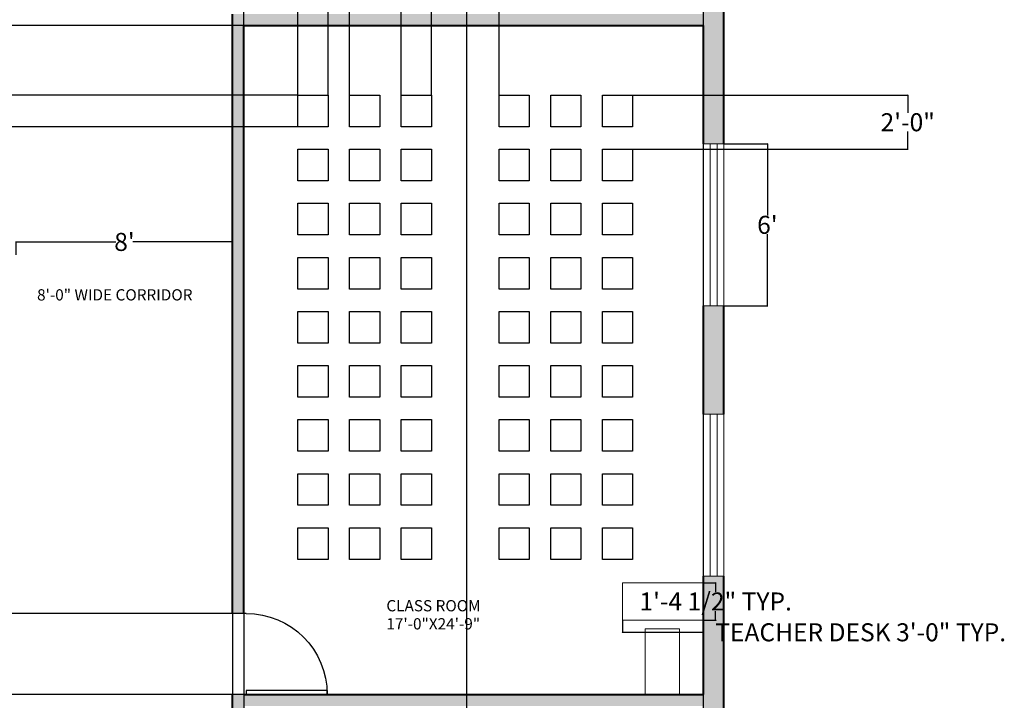
# Model space of a CAD drawing. Units: inches. Extents: x -405 to 940, y 226 to 2032.
# Tile 9 of 10: x 503 to 940, y 1301 to 1603. Entities that reach past the tile are written whole.
import ezdxf

# ---------------------------------------------------------------- set-up
doc = ezdxf.new("R2010")
doc.units = ezdxf.units.IN
doc.header["$MEASUREMENT"] = 0
doc.linetypes.add('ACAD_ISO02W100', pattern=[15, 12, -3])
for name, color, linetype, lineweight in [('A-ANNO-DIMS', 120, 'Continuous', 18), ('A-AREA-IDEN', 32, 'Continuous', 18), ('A-FURN-SEAT', 5, 'Continuous', 18), ('A-GLAZ-HIDN', 1, 'ACAD_ISO02W100', 18), ('A-WALL-PATT', 8, 'Continuous', 13), ('door', 6, 'Continuous', 25), ('tables', 2, 'Continuous', 18), ('wall', 3, 'Continuous', 40), ('window', 1, 'Continuous', 18)]:
    doc.layers.add(name, color=color, linetype=linetype, lineweight=lineweight)
doc.layers.add('beches', color=5, linetype='Continuous')
doc.styles.get("Standard").update_dxf_attribs({"font": 'arial.ttf'})
doc.dimstyles.get("Standard").update_dxf_attribs({"dimtxt": 8, "dimasz": 0.18, "dimexe": 0.18, "dimexo": 0.0625, "dimgap": 0.09, "dimtad": 0, "dimtih": 1, "dimtoh": 1, "dimdec": 0, "dimzin": 0, "dimdsep": 46, "dimlunit": 3, "dimtxsty": 'Standard', "dimblk": 'OBLIQUE', "dimcen": 0.09, "dimadec": 0, "dimazin": 0, "dimtfac": 1, "dimtdec": 0, "dimtofl": 0, "dimtmove": 0, "dimatfit": 3, "dimfxl": 1, "dimtolj": 1, "dimtzin": 0, "dimarcsym": 0})

# ---------------------------------------------------------------- blocks, each defined once
blk = doc.blocks.new('*U4')
for p, q in [((0, 0), (0, -6)), ((36, 0), (36, -6))]:
    blk.add_line(p, q)
blk.add_lwpolyline([(0, 0), (0, 36), (1.75, 36), (1.75, 0)], close=True)
blk.add_arc((0, 0), 36, 0, 90)
blk = doc.blocks.new('*U25')
at = {"layer": 'beches'}
blk.add_lwpolyline([(6.71, -7.02), (-6.71, -7.02), (-6.71, 7.02), (6.71, 7.02)], close=True, dxfattribs=at)
blk = doc.blocks.new('*U26')
at = {"layer": 'A-FURN-SEAT', "transparency": 16777216}
for p in [(-45.84, 192), (-45.84, 192, 12), (-45.84, 192, 24), (-45.84, 192, 36), (-45.84, 192, 48), (-45.84, 192, 60), (-45.84, 192, 72), (-45.84, 192, 84), (-45.84, 192, 96), (-45.84, 192, 108), (-45.84, 192, 120), (-45.84, 192, 132), (-22.92, 192), (-22.92, 192, 12), (-22.92, 192, 24), (-22.92, 192, 36), (-22.92, 192, 48), (-22.92, 192, 60), (-22.92, 192, 72), (-22.92, 192, 84), (-22.92, 192, 96), (-22.92, 192, 108), (-22.92, 192, 120), (-22.92, 192, 132), (0, 192), (0, 192, 12), (0, 192, 24), (0, 192, 36), (0, 192, 48), (0, 192, 60), (0, 192, 72), (0, 192, 84), (0, 192, 96), (0, 192, 108), (0, 192, 120), (0, 192, 132), (-45.84, 168), (-45.84, 168, 12), (-45.84, 168, 24), (-45.84, 168, 36), (-45.84, 168, 48), (-45.84, 168, 60), (-45.84, 168, 72), (-45.84, 168, 84), (-45.84, 168, 96), (-45.84, 168, 108), (-45.84, 168, 120), (-45.84, 168, 132), (-22.92, 168), (-22.92, 168, 12), (-22.92, 168, 24), (-22.92, 168, 36), (-22.92, 168, 48), (-22.92, 168, 60), (-22.92, 168, 72), (-22.92, 168, 84), (-22.92, 168, 96), (-22.92, 168, 108), (-22.92, 168, 120), (-22.92, 168, 132), (0, 168), (0, 168, 12), (0, 168, 24), (0, 168, 36), (0, 168, 48), (0, 168, 60), (0, 168, 72), (0, 168, 84), (0, 168, 96), (0, 168, 108), (0, 168, 120), (0, 168, 132), (-45.84, 144), (-45.84, 144, 12), (-45.84, 144, 24), (-45.84, 144, 36), (-45.84, 144, 48), (-45.84, 144, 60), (-45.84, 144, 72), (-45.84, 144, 84), (-45.84, 144, 96), (-45.84, 144, 108), (-45.84, 144, 120), (-45.84, 144, 132), (-22.92, 144), (-22.92, 144, 12), (-22.92, 144, 24), (-22.92, 144, 36), (-22.92, 144, 48), (-22.92, 144, 60), (-22.92, 144, 72), (-22.92, 144, 84), (-22.92, 144, 96), (-22.92, 144, 108), (-22.92, 144, 120), (-22.92, 144, 132), (0, 144), (0, 144, 12), (0, 144, 24), (0, 144, 36), (0, 144, 48), (0, 144, 60), (0, 144, 72), (0, 144, 84), (0, 144, 96), (0, 144, 108), (0, 144, 120), (0, 144, 132), (-45.84, 120), (-45.84, 120, 12), (-45.84, 120, 24), (-45.84, 120, 36), (-45.84, 120, 48), (-45.84, 120, 60), (-45.84, 120, 72), (-45.84, 120, 84), (-45.84, 120, 96), (-45.84, 120, 108), (-45.84, 120, 120), (-45.84, 120, 132), (-22.92, 120), (-22.92, 120, 12), (-22.92, 120, 24), (-22.92, 120, 36), (-22.92, 120, 48), (-22.92, 120, 60), (-22.92, 120, 72), (-22.92, 120, 84), (-22.92, 120, 96), (-22.92, 120, 108), (-22.92, 120, 120), (-22.92, 120, 132), (0, 120), (0, 120, 12), (0, 120, 24), (0, 120, 36), (0, 120, 48), (0, 120, 60), (0, 120, 72), (0, 120, 84), (0, 120, 96), (0, 120, 108), (0, 120, 120), (0, 120, 132), (-45.84, 96), (-45.84, 96, 12), (-45.84, 96, 24), (-45.84, 96, 36), (-45.84, 96, 48), (-45.84, 96, 60), (-45.84, 96, 72), (-45.84, 96, 84), (-45.84, 96, 96), (-45.84, 96, 108), (-45.84, 96, 120), (-45.84, 96, 132), (-22.92, 96), (-22.92, 96, 12), (-22.92, 96, 24), (-22.92, 96, 36), (-22.92, 96, 48), (-22.92, 96, 60), (-22.92, 96, 72), (-22.92, 96, 84), (-22.92, 96, 96), (-22.92, 96, 108), (-22.92, 96, 120), (-22.92, 96, 132), (0, 96), (0, 96, 12), (0, 96, 24), (0, 96, 36), (0, 96, 48), (0, 96, 60), (0, 96, 72), (0, 96, 84), (0, 96, 96), (0, 96, 108), (0, 96, 120), (0, 96, 132), (-45.84, 72), (-45.84, 72, 12), (-45.84, 72, 24), (-45.84, 72, 36), (-45.84, 72, 48), (-45.84, 72, 60), (-45.84, 72, 72), (-45.84, 72, 84), (-45.84, 72, 96), (-45.84, 72, 108), (-45.84, 72, 120), (-45.84, 72, 132), (-22.92, 72), (-22.92, 72, 12), (-22.92, 72, 24), (-22.92, 72, 36), (-22.92, 72, 48), (-22.92, 72, 60), (-22.92, 72, 72), (-22.92, 72, 84), (-22.92, 72, 96), (-22.92, 72, 108), (-22.92, 72, 120), (-22.92, 72, 132), (0, 72), (0, 72, 12), (0, 72, 24), (0, 72, 36), (0, 72, 48), (0, 72, 60), (0, 72, 72), (0, 72, 84), (0, 72, 96), (0, 72, 108), (0, 72, 120), (0, 72, 132), (-45.84, 48), (-45.84, 48, 12), (-45.84, 48, 24), (-45.84, 48, 36), (-45.84, 48, 48), (-45.84, 48, 60), (-45.84, 48, 72), (-45.84, 48, 84), (-45.84, 48, 96), (-45.84, 48, 108), (-45.84, 48, 120), (-45.84, 48, 132), (-22.92, 48), (-22.92, 48, 12), (-22.92, 48, 24), (-22.92, 48, 36), (-22.92, 48, 48), (-22.92, 48, 60), (-22.92, 48, 72), (-22.92, 48, 84), (-22.92, 48, 96), (-22.92, 48, 108), (-22.92, 48, 120), (-22.92, 48, 132), (0, 48), (0, 48, 12), (0, 48, 24), (0, 48, 36), (0, 48, 48), (0, 48, 60), (0, 48, 72), (0, 48, 84), (0, 48, 96), (0, 48, 108), (0, 48, 120), (0, 48, 132), (-45.84, 24), (-45.84, 24, 12), (-45.84, 24, 24), (-45.84, 24, 36), (-45.84, 24, 48), (-45.84, 24, 60), (-45.84, 24, 72), (-45.84, 24, 84), (-45.84, 24, 96), (-45.84, 24, 108), (-45.84, 24, 120), (-45.84, 24, 132), (-22.92, 24), (-22.92, 24, 12), (-22.92, 24, 24), (-22.92, 24, 36), (-22.92, 24, 48), (-22.92, 24, 60), (-22.92, 24, 72), (-22.92, 24, 84), (-22.92, 24, 96), (-22.92, 24, 108), (-22.92, 24, 120), (-22.92, 24, 132), (0, 24), (0, 24, 12), (0, 24, 24), (0, 24, 36), (0, 24, 48), (0, 24, 60), (0, 24, 72), (0, 24, 84), (0, 24, 96), (0, 24, 108), (0, 24, 120), (0, 24, 132), (-45.84, 0), (-45.84, 0, 12), (-45.84, 0, 24), (-45.84, 0, 36), (-45.84, 0, 48), (-45.84, 0, 60), (-45.84, 0, 72), (-45.84, 0, 84), (-45.84, 0, 96), (-45.84, 0, 108), (-45.84, 0, 120), (-45.84, 0, 132), (-22.92, 0), (-22.92, 0, 12), (-22.92, 0, 24), (-22.92, 0, 36), (-22.92, 0, 48), (-22.92, 0, 60), (-22.92, 0, 72), (-22.92, 0, 84), (-22.92, 0, 96), (-22.92, 0, 108), (-22.92, 0, 120), (-22.92, 0, 132), (0, 0), (0, 0, 12), (0, 0, 24), (0, 0, 36), (0, 0, 48), (0, 0, 60), (0, 0, 72), (0, 0, 84), (0, 0, 96), (0, 0, 108), (0, 0, 120), (0, 0, 132)]:
    blk.add_blockref('*U25', p, dxfattribs=at)
blk = doc.blocks.new('*U23')
at = {"layer": 'beches'}
blk.add_lwpolyline([(6.71, -7.02), (-6.71, -7.02), (-6.71, 7.02), (6.71, 7.02)], close=True, dxfattribs=at)
blk = doc.blocks.new('*U24')
at = {"layer": 'A-FURN-SEAT', "transparency": 16777216}
for p in [(-45.84, 192), (-45.84, 192, 12), (-45.84, 192, 24), (-45.84, 192, 36), (-45.84, 192, 48), (-45.84, 192, 60), (-45.84, 192, 72), (-45.84, 192, 84), (-45.84, 192, 96), (-45.84, 192, 108), (-45.84, 192, 120), (-45.84, 192, 132), (-22.92, 192), (-22.92, 192, 12), (-22.92, 192, 24), (-22.92, 192, 36), (-22.92, 192, 48), (-22.92, 192, 60), (-22.92, 192, 72), (-22.92, 192, 84), (-22.92, 192, 96), (-22.92, 192, 108), (-22.92, 192, 120), (-22.92, 192, 132), (0, 192), (0, 192, 12), (0, 192, 24), (0, 192, 36), (0, 192, 48), (0, 192, 60), (0, 192, 72), (0, 192, 84), (0, 192, 96), (0, 192, 108), (0, 192, 120), (0, 192, 132), (-45.84, 168), (-45.84, 168, 12), (-45.84, 168, 24), (-45.84, 168, 36), (-45.84, 168, 48), (-45.84, 168, 60), (-45.84, 168, 72), (-45.84, 168, 84), (-45.84, 168, 96), (-45.84, 168, 108), (-45.84, 168, 120), (-45.84, 168, 132), (-22.92, 168), (-22.92, 168, 12), (-22.92, 168, 24), (-22.92, 168, 36), (-22.92, 168, 48), (-22.92, 168, 60), (-22.92, 168, 72), (-22.92, 168, 84), (-22.92, 168, 96), (-22.92, 168, 108), (-22.92, 168, 120), (-22.92, 168, 132), (0, 168), (0, 168, 12), (0, 168, 24), (0, 168, 36), (0, 168, 48), (0, 168, 60), (0, 168, 72), (0, 168, 84), (0, 168, 96), (0, 168, 108), (0, 168, 120), (0, 168, 132), (-45.84, 144), (-45.84, 144, 12), (-45.84, 144, 24), (-45.84, 144, 36), (-45.84, 144, 48), (-45.84, 144, 60), (-45.84, 144, 72), (-45.84, 144, 84), (-45.84, 144, 96), (-45.84, 144, 108), (-45.84, 144, 120), (-45.84, 144, 132), (-22.92, 144), (-22.92, 144, 12), (-22.92, 144, 24), (-22.92, 144, 36), (-22.92, 144, 48), (-22.92, 144, 60), (-22.92, 144, 72), (-22.92, 144, 84), (-22.92, 144, 96), (-22.92, 144, 108), (-22.92, 144, 120), (-22.92, 144, 132), (0, 144), (0, 144, 12), (0, 144, 24), (0, 144, 36), (0, 144, 48), (0, 144, 60), (0, 144, 72), (0, 144, 84), (0, 144, 96), (0, 144, 108), (0, 144, 120), (0, 144, 132), (-45.84, 120), (-45.84, 120, 12), (-45.84, 120, 24), (-45.84, 120, 36), (-45.84, 120, 48), (-45.84, 120, 60), (-45.84, 120, 72), (-45.84, 120, 84), (-45.84, 120, 96), (-45.84, 120, 108), (-45.84, 120, 120), (-45.84, 120, 132), (-22.92, 120), (-22.92, 120, 12), (-22.92, 120, 24), (-22.92, 120, 36), (-22.92, 120, 48), (-22.92, 120, 60), (-22.92, 120, 72), (-22.92, 120, 84), (-22.92, 120, 96), (-22.92, 120, 108), (-22.92, 120, 120), (-22.92, 120, 132), (0, 120), (0, 120, 12), (0, 120, 24), (0, 120, 36), (0, 120, 48), (0, 120, 60), (0, 120, 72), (0, 120, 84), (0, 120, 96), (0, 120, 108), (0, 120, 120), (0, 120, 132), (-45.84, 96), (-45.84, 96, 12), (-45.84, 96, 24), (-45.84, 96, 36), (-45.84, 96, 48), (-45.84, 96, 60), (-45.84, 96, 72), (-45.84, 96, 84), (-45.84, 96, 96), (-45.84, 96, 108), (-45.84, 96, 120), (-45.84, 96, 132), (-22.92, 96), (-22.92, 96, 12), (-22.92, 96, 24), (-22.92, 96, 36), (-22.92, 96, 48), (-22.92, 96, 60), (-22.92, 96, 72), (-22.92, 96, 84), (-22.92, 96, 96), (-22.92, 96, 108), (-22.92, 96, 120), (-22.92, 96, 132), (0, 96), (0, 96, 12), (0, 96, 24), (0, 96, 36), (0, 96, 48), (0, 96, 60), (0, 96, 72), (0, 96, 84), (0, 96, 96), (0, 96, 108), (0, 96, 120), (0, 96, 132), (-45.84, 72), (-45.84, 72, 12), (-45.84, 72, 24), (-45.84, 72, 36), (-45.84, 72, 48), (-45.84, 72, 60), (-45.84, 72, 72), (-45.84, 72, 84), (-45.84, 72, 96), (-45.84, 72, 108), (-45.84, 72, 120), (-45.84, 72, 132), (-22.92, 72), (-22.92, 72, 12), (-22.92, 72, 24), (-22.92, 72, 36), (-22.92, 72, 48), (-22.92, 72, 60), (-22.92, 72, 72), (-22.92, 72, 84), (-22.92, 72, 96), (-22.92, 72, 108), (-22.92, 72, 120), (-22.92, 72, 132), (0, 72), (0, 72, 12), (0, 72, 24), (0, 72, 36), (0, 72, 48), (0, 72, 60), (0, 72, 72), (0, 72, 84), (0, 72, 96), (0, 72, 108), (0, 72, 120), (0, 72, 132), (-45.84, 48), (-45.84, 48, 12), (-45.84, 48, 24), (-45.84, 48, 36), (-45.84, 48, 48), (-45.84, 48, 60), (-45.84, 48, 72), (-45.84, 48, 84), (-45.84, 48, 96), (-45.84, 48, 108), (-45.84, 48, 120), (-45.84, 48, 132), (-22.92, 48), (-22.92, 48, 12), (-22.92, 48, 24), (-22.92, 48, 36), (-22.92, 48, 48), (-22.92, 48, 60), (-22.92, 48, 72), (-22.92, 48, 84), (-22.92, 48, 96), (-22.92, 48, 108), (-22.92, 48, 120), (-22.92, 48, 132), (0, 48), (0, 48, 12), (0, 48, 24), (0, 48, 36), (0, 48, 48), (0, 48, 60), (0, 48, 72), (0, 48, 84), (0, 48, 96), (0, 48, 108), (0, 48, 120), (0, 48, 132), (-45.84, 24), (-45.84, 24, 12), (-45.84, 24, 24), (-45.84, 24, 36), (-45.84, 24, 48), (-45.84, 24, 60), (-45.84, 24, 72), (-45.84, 24, 84), (-45.84, 24, 96), (-45.84, 24, 108), (-45.84, 24, 120), (-45.84, 24, 132), (-22.92, 24), (-22.92, 24, 12), (-22.92, 24, 24), (-22.92, 24, 36), (-22.92, 24, 48), (-22.92, 24, 60), (-22.92, 24, 72), (-22.92, 24, 84), (-22.92, 24, 96), (-22.92, 24, 108), (-22.92, 24, 120), (-22.92, 24, 132), (0, 24), (0, 24, 12), (0, 24, 24), (0, 24, 36), (0, 24, 48), (0, 24, 60), (0, 24, 72), (0, 24, 84), (0, 24, 96), (0, 24, 108), (0, 24, 120), (0, 24, 132), (-45.84, 0), (-45.84, 0, 12), (-45.84, 0, 24), (-45.84, 0, 36), (-45.84, 0, 48), (-45.84, 0, 60), (-45.84, 0, 72), (-45.84, 0, 84), (-45.84, 0, 96), (-45.84, 0, 108), (-45.84, 0, 120), (-45.84, 0, 132), (-22.92, 0), (-22.92, 0, 12), (-22.92, 0, 24), (-22.92, 0, 36), (-22.92, 0, 48), (-22.92, 0, 60), (-22.92, 0, 72), (-22.92, 0, 84), (-22.92, 0, 96), (-22.92, 0, 108), (-22.92, 0, 120), (-22.92, 0, 132), (0, 0), (0, 0, 12), (0, 0, 24), (0, 0, 36), (0, 0, 48), (0, 0, 60), (0, 0, 72), (0, 0, 84), (0, 0, 96), (0, 0, 108), (0, 0, 120), (0, 0, 132)]:
    blk.add_blockref('*U23', p, dxfattribs=at)
blk = doc.blocks.new('_Oblique')
at = {"color": 0, "linetype": 'ByBlock', "lineweight": -2}
blk.add_line((-0.5, -0.5), (0.5, 0.5), dxfattribs=at)
blk = doc.blocks.new('*D42')
at = {"layer": 'A-ANNO-DIMS', "color": 0, "lineweight": -2, "transparency": 16777216}
for p, q in [((501.77, 1498.93), (501.77, 1504.9)), ((501.77, 1504.72), (545.99, 1504.72)), ((597.77, 1504.72), (553.54, 1504.72)), ((597.77, 1498.93), (597.77, 1504.9))]:
    blk.add_line(p, q, dxfattribs=at)
at = {"layer": 'Defpoints', "color": 0, "transparency": 16777216}
for p in [(501.77, 1504.72), (501.77, 1498.87), (597.77, 1498.87)]:
    blk.add_point(p, dxfattribs=at)
at = {"layer": 'A-ANNO-DIMS', "color": 0, "lineweight": -2, "transparency": 16777216, "xscale": 0.18, "yscale": 0.18, "zscale": 0.18, "rotation": 180}
blk.add_blockref('_Oblique', (501.77, 1504.72), dxfattribs=at)
at = {"layer": 'A-ANNO-DIMS', "color": 0, "lineweight": -2, "transparency": 16777216, "xscale": 0.18, "yscale": 0.18, "zscale": 0.18}
blk.add_blockref('_Oblique', (597.77, 1504.72), dxfattribs=at)
at = {"layer": 'A-ANNO-DIMS', "color": 0, "transparency": 16777216, "insert": (549.77, 1504.72), "char_height": 8, "attachment_point": 5}
blk.add_mtext("\\A1;8'", dxfattribs=at)
blk = doc.blocks.new('*D69')
at = {"layer": 'A-ANNO-DIMS', "color": 0, "lineweight": -2, "transparency": 16777216}
for p, q in [((815.83, 1548.31), (835.31, 1548.31)), ((835.13, 1548.31), (835.13, 1516.48)), ((835.13, 1476.31), (835.13, 1508.14)), ((815.83, 1476.31), (835.31, 1476.31))]:
    blk.add_line(p, q, dxfattribs=at)
at = {"layer": 'Defpoints', "color": 0, "transparency": 16777216}
for p in [(815.77, 1548.31), (815.77, 1476.31), (835.13, 1476.31)]:
    blk.add_point(p, dxfattribs=at)
at = {"layer": 'A-ANNO-DIMS', "color": 0, "lineweight": -2, "transparency": 16777216, "xscale": 0.18, "yscale": 0.18, "zscale": 0.18}
for p, rotation in [((835.13, 1548.31), 90), ((835.13, 1476.31), 270)]:
    blk.add_blockref('_Oblique', p, dxfattribs=dict(at, rotation=rotation))
at = {"layer": 'A-ANNO-DIMS', "color": 0, "transparency": 16777216, "insert": (835.13, 1512.31), "char_height": 8, "attachment_point": 5}
blk.add_mtext("\\A1;6'", dxfattribs=at)
blk = doc.blocks.new('CLASSROOM-DESK-WIDE')
for p, q in [((0, 0), (0, 16.56)), ((0, 16.56), (36, 16.56)), ((36, 16.56), (36, 0)), ((36, 0), (0, 0))]:
    blk.add_line(p, q)
blk = doc.blocks.new('CHAIR-DESK')
blk.add_lwpolyline([(0, 15.21), (28.97, 15.21), (28.97, 0), (0, 0)], close=True)
blk = doc.blocks.new('WIN-PANE-72IN')
for p, q in [((0, 3), (72, 3)), ((0, 0), (72, 0))]:
    blk.add_line(p, q)
blk = doc.blocks.new('*D95')
at = {"layer": 'A-ANNO-DIMS', "color": 0, "lineweight": -2, "transparency": 16777216}
for p, q in [((770.77, 1336.78), (770.77, 1331.27)), ((806.77, 1336.78), (806.77, 1331.27)), ((770.77, 1331.45), (806.77, 1331.45)), ((806.77, 1331.45), (806.95, 1331.45))]:
    blk.add_line(p, q, dxfattribs=at)
at = {"layer": 'Defpoints', "color": 0, "transparency": 16777216}
for p in [(770.77, 1336.85), (806.77, 1336.85), (806.77, 1331.45)]:
    blk.add_point(p, dxfattribs=at)
at = {"layer": 'A-ANNO-DIMS', "color": 0, "lineweight": -2, "transparency": 16777216, "xscale": 0.18, "yscale": 0.18, "zscale": 0.18, "rotation": 180}
blk.add_blockref('_Oblique', (770.77, 1331.45), dxfattribs=at)
at = {"layer": 'A-ANNO-DIMS', "color": 0, "lineweight": -2, "transparency": 16777216, "xscale": 0.18, "yscale": 0.18, "zscale": 0.18}
blk.add_blockref('_Oblique', (806.77, 1331.45), dxfattribs=at)
at = {"layer": 'A-ANNO-DIMS', "color": 0, "transparency": 16777216, "insert": (876.54, 1331.45), "char_height": 8, "attachment_point": 5}
blk.add_mtext('\\A1;TEACHER DESK 3\'-0" TYP.', dxfattribs=at)
blk = doc.blocks.new('*D96')
at = {"layer": 'A-ANNO-DIMS', "color": 0, "lineweight": -2, "transparency": 16777216}
for p, q in [((806.83, 1353.41), (812.35, 1353.41)), ((812.17, 1353.41), (812.17, 1349.35)), ((812.17, 1336.85), (812.17, 1340.9)), ((806.83, 1336.85), (812.35, 1336.85))]:
    blk.add_line(p, q, dxfattribs=at)
at = {"layer": 'Defpoints', "color": 0, "transparency": 16777216}
for p in [(806.77, 1353.41), (812.17, 1353.41), (806.77, 1336.85)]:
    blk.add_point(p, dxfattribs=at)
at = {"layer": 'A-ANNO-DIMS', "color": 0, "lineweight": -2, "transparency": 16777216, "xscale": 0.18, "yscale": 0.18, "zscale": 0.18}
for p, rotation in [((812.17, 1353.41), 90), ((812.17, 1336.85), 270)]:
    blk.add_blockref('_Oblique', p, dxfattribs=dict(at, rotation=rotation))
at = {"layer": 'A-ANNO-DIMS', "color": 0, "transparency": 16777216, "insert": (812.17, 1345.13), "char_height": 8, "attachment_point": 5}
blk.add_mtext('\\A1;1\'-4 1/2" TYP.', dxfattribs=at)
blk = doc.blocks.new('*D99')
at = {"layer": 'A-ANNO-DIMS', "color": 0, "lineweight": -2, "transparency": 16777216}
for p, q in [((626.77, 1569.91), (626.77, 2020.64)), ((626.77, 2020.46), (640.19, 2020.46)), ((640.19, 1569.91), (640.19, 2020.64)), ((640.19, 2020.46), (640.37, 2020.46))]:
    blk.add_line(p, q, dxfattribs=at)
at = {"layer": 'Defpoints', "color": 0, "transparency": 16777216}
for p in [(640.19, 2020.46), (626.77, 1569.84), (640.19, 1569.84)]:
    blk.add_point(p, dxfattribs=at)
at = {"layer": 'A-ANNO-DIMS', "color": 0, "lineweight": -2, "transparency": 16777216, "xscale": 0.18, "yscale": 0.18, "zscale": 0.18, "rotation": 180}
blk.add_blockref('_Oblique', (626.77, 2020.46), dxfattribs=at)
at = {"layer": 'A-ANNO-DIMS', "color": 0, "lineweight": -2, "transparency": 16777216, "xscale": 0.18, "yscale": 0.18, "zscale": 0.18}
blk.add_blockref('_Oblique', (640.19, 2020.46), dxfattribs=at)
at = {"layer": 'A-ANNO-DIMS', "color": 0, "transparency": 16777216, "insert": (660.04, 2020.46), "char_height": 8, "attachment_point": 5}
blk.add_mtext('\\A1;1\'-1 1/2"', dxfattribs=at)
blk = doc.blocks.new('*D100')
at = {"layer": 'A-ANNO-DIMS', "color": 0, "lineweight": -2, "transparency": 16777216}
for p, q in [((626.71, 1569.84), (-390.06, 1569.84)), ((-389.88, 1569.84), (-389.88, 1566.93)), ((626.71, 1555.81), (-390.06, 1555.81)), ((-389.88, 1555.81), (-389.88, 1558.72))]:
    blk.add_line(p, q, dxfattribs=at)
at = {"layer": 'Defpoints', "color": 0, "transparency": 16777216}
for p in [(626.77, 1569.84), (-389.88, 1555.81), (626.77, 1555.81)]:
    blk.add_point(p, dxfattribs=at)
at = {"layer": 'A-ANNO-DIMS', "color": 0, "lineweight": -2, "transparency": 16777216, "xscale": 0.18, "yscale": 0.18, "zscale": 0.18}
for p, rotation in [((-389.88, 1569.84), 90), ((-389.88, 1555.81), 270)]:
    blk.add_blockref('_Oblique', p, dxfattribs=dict(at, rotation=rotation))
at = {"layer": 'A-ANNO-DIMS', "color": 0, "transparency": 16777216, "insert": (-389.88, 1562.83), "char_height": 8, "attachment_point": 5}
blk.add_mtext('\\A1;1\'-2"', dxfattribs=at)
blk = doc.blocks.new('*D101')
at = {"layer": 'A-ANNO-DIMS', "color": 0, "lineweight": -2, "transparency": 16777216}
for p, q in [((649.69, 1569.91), (649.69, 2020.64)), ((649.69, 2020.46), (672.61, 2020.46)), ((672.61, 1569.91), (672.61, 2020.64)), ((672.61, 2020.46), (672.79, 2020.46))]:
    blk.add_line(p, q, dxfattribs=at)
at = {"layer": 'Defpoints', "color": 0, "transparency": 16777216}
for p in [(672.61, 2020.46), (649.69, 1569.84), (672.61, 1569.84)]:
    blk.add_point(p, dxfattribs=at)
at = {"layer": 'A-ANNO-DIMS', "color": 0, "lineweight": -2, "transparency": 16777216, "xscale": 0.18, "yscale": 0.18, "zscale": 0.18, "rotation": 180}
blk.add_blockref('_Oblique', (649.69, 2020.46), dxfattribs=at)
at = {"layer": 'A-ANNO-DIMS', "color": 0, "lineweight": -2, "transparency": 16777216, "xscale": 0.18, "yscale": 0.18, "zscale": 0.18}
blk.add_blockref('_Oblique', (672.61, 2020.46), dxfattribs=at)
at = {"layer": 'A-ANNO-DIMS', "color": 0, "transparency": 16777216, "insert": (686.25, 2020.46), "char_height": 8, "attachment_point": 5}
blk.add_mtext('\\A1;1\'-11"', dxfattribs=at)
blk = doc.blocks.new('*D102')
at = {"layer": 'A-ANNO-DIMS', "color": 0, "lineweight": -2, "transparency": 16777216}
for p, q in [((775.36, 1569.84), (897.6, 1569.84)), ((897.42, 1569.84), (897.42, 1562.02)), ((897.42, 1545.84), (897.42, 1553.67)), ((775.36, 1545.84), (897.6, 1545.84))]:
    blk.add_line(p, q, dxfattribs=at)
at = {"layer": 'Defpoints', "color": 0, "transparency": 16777216}
for p in [(775.3, 1569.84), (775.3, 1545.84), (897.42, 1545.84)]:
    blk.add_point(p, dxfattribs=at)
at = {"layer": 'A-ANNO-DIMS', "color": 0, "lineweight": -2, "transparency": 16777216, "xscale": 0.18, "yscale": 0.18, "zscale": 0.18}
for p, rotation in [((897.42, 1569.84), 90), ((897.42, 1545.84), 270)]:
    blk.add_blockref('_Oblique', p, dxfattribs=dict(at, rotation=rotation))
at = {"layer": 'A-ANNO-DIMS', "color": 0, "transparency": 16777216, "insert": (897.42, 1557.84), "char_height": 8, "attachment_point": 5}
blk.add_mtext('\\A1;2\'-0"', dxfattribs=at)
blk = doc.blocks.new('*D103')
at = {"layer": 'A-ANNO-DIMS', "color": 0, "lineweight": -2, "transparency": 16777216}
for p, q in [((686.03, 1569.91), (686.03, 2020.64)), ((686.03, 2020.46), (690.24, 2020.46)), ((716.03, 2020.46), (711.82, 2020.46)), ((716.03, 1569.91), (716.03, 2020.64))]:
    blk.add_line(p, q, dxfattribs=at)
at = {"layer": 'Defpoints', "color": 0, "transparency": 16777216}
for p in [(716.03, 2020.46), (686.03, 1569.84), (716.03, 1569.84)]:
    blk.add_point(p, dxfattribs=at)
at = {"layer": 'A-ANNO-DIMS', "color": 0, "lineweight": -2, "transparency": 16777216, "xscale": 0.18, "yscale": 0.18, "zscale": 0.18, "rotation": 180}
blk.add_blockref('_Oblique', (686.03, 2020.46), dxfattribs=at)
at = {"layer": 'A-ANNO-DIMS', "color": 0, "lineweight": -2, "transparency": 16777216, "xscale": 0.18, "yscale": 0.18, "zscale": 0.18}
blk.add_blockref('_Oblique', (716.03, 2020.46), dxfattribs=at)
at = {"layer": 'A-ANNO-DIMS', "color": 0, "transparency": 16777216, "insert": (701.03, 2020.46), "char_height": 8, "attachment_point": 5}
blk.add_mtext('\\A1;2\'-6"', dxfattribs=at)
blk = doc.blocks.new('*D104')
at = {"layer": 'A-ANNO-DIMS', "color": 0, "lineweight": -2, "transparency": 16777216}
for p, q in [((602.77, 1600.87), (602.77, 2020.64)), ((602.77, 2020.46), (603.98, 2020.46)), ((626.77, 2020.46), (625.56, 2020.46)), ((626.77, 1569.91), (626.77, 2020.64))]:
    blk.add_line(p, q, dxfattribs=at)
at = {"layer": 'Defpoints', "color": 0, "transparency": 16777216}
for p in [(626.77, 2020.46), (602.77, 1600.81), (626.77, 1569.84)]:
    blk.add_point(p, dxfattribs=at)
at = {"layer": 'A-ANNO-DIMS', "color": 0, "lineweight": -2, "transparency": 16777216, "xscale": 0.18, "yscale": 0.18, "zscale": 0.18, "rotation": 180}
blk.add_blockref('_Oblique', (602.77, 2020.46), dxfattribs=at)
at = {"layer": 'A-ANNO-DIMS', "color": 0, "lineweight": -2, "transparency": 16777216, "xscale": 0.18, "yscale": 0.18, "zscale": 0.18}
blk.add_blockref('_Oblique', (626.77, 2020.46), dxfattribs=at)
at = {"layer": 'A-ANNO-DIMS', "color": 0, "transparency": 16777216, "insert": (614.77, 2020.46), "char_height": 8, "attachment_point": 5}
blk.add_mtext('\\A1;2\'-0"', dxfattribs=at)
blk = doc.blocks.new('*D105')
at = {"layer": 'A-ANNO-DIMS', "color": 0, "lineweight": -2, "transparency": 16777216}
for p, q in [((602.71, 1600.81), (-390.06, 1600.81)), ((-389.88, 1600.81), (-389.88, 1589.43)), ((-389.88, 1569.84), (-389.88, 1581.22)), ((626.71, 1569.84), (-390.06, 1569.84))]:
    blk.add_line(p, q, dxfattribs=at)
at = {"layer": 'Defpoints', "color": 0, "transparency": 16777216}
for p in [(602.77, 1600.81), (-389.88, 1569.84), (626.77, 1569.84)]:
    blk.add_point(p, dxfattribs=at)
at = {"layer": 'A-ANNO-DIMS', "color": 0, "lineweight": -2, "transparency": 16777216, "xscale": 0.18, "yscale": 0.18, "zscale": 0.18}
for p, rotation in [((-389.88, 1600.81), 90), ((-389.88, 1569.84), 270)]:
    blk.add_blockref('_Oblique', p, dxfattribs=dict(at, rotation=rotation))
at = {"layer": 'A-ANNO-DIMS', "color": 0, "transparency": 16777216, "insert": (-389.88, 1585.33), "char_height": 8, "attachment_point": 5}
blk.add_mtext('\\A1;2\'-7"', dxfattribs=at)
blk = doc.blocks.new('*D112')
at = {"layer": 'A-ANNO-DIMS', "color": 0, "lineweight": -2, "transparency": 16777216}
for p, q in [((701.77, 534.87), (701.77, 2020.64)), ((701.77, 2020.46), (743.54, 2020.46)), ((806.77, 2020.46), (765, 2020.46)), ((806.77, 534.87), (806.77, 2020.64))]:
    blk.add_line(p, q, dxfattribs=at)
at = {"layer": 'Defpoints', "color": 0, "transparency": 16777216}
for p in [(701.77, 2020.46), (701.77, 534.81), (806.77, 534.81)]:
    blk.add_point(p, dxfattribs=at)
at = {"layer": 'A-ANNO-DIMS', "color": 0, "lineweight": -2, "transparency": 16777216, "xscale": 0.18, "yscale": 0.18, "zscale": 0.18, "rotation": 180}
blk.add_blockref('_Oblique', (701.77, 2020.46), dxfattribs=at)
at = {"layer": 'A-ANNO-DIMS', "color": 0, "lineweight": -2, "transparency": 16777216, "xscale": 0.18, "yscale": 0.18, "zscale": 0.18}
blk.add_blockref('_Oblique', (806.77, 2020.46), dxfattribs=at)
at = {"layer": 'A-ANNO-DIMS', "color": 0, "transparency": 16777216, "insert": (754.27, 2020.46), "char_height": 8, "attachment_point": 5}
blk.add_mtext('\\A1;8\'-9"', dxfattribs=at)
blk = doc.blocks.new('*D114')
at = {"layer": 'A-ANNO-DIMS', "color": 0, "lineweight": -2, "transparency": 16777216}
for p, q in [((602.71, 1339.81), (-390.06, 1339.81)), ((-389.88, 1339.81), (-389.88, 1325.99)), ((-389.88, 1303.81), (-389.88, 1317.63)), ((602.71, 1303.81), (-390.06, 1303.81))]:
    blk.add_line(p, q, dxfattribs=at)
at = {"layer": 'Defpoints', "color": 0, "transparency": 16777216}
for p in [(602.77, 1339.81), (-389.88, 1303.81), (602.77, 1303.81)]:
    blk.add_point(p, dxfattribs=at)
at = {"layer": 'A-ANNO-DIMS', "color": 0, "lineweight": -2, "transparency": 16777216, "xscale": 0.18, "yscale": 0.18, "zscale": 0.18}
for p, rotation in [((-389.88, 1339.81), 90), ((-389.88, 1303.81), 270)]:
    blk.add_blockref('_Oblique', p, dxfattribs=dict(at, rotation=rotation))
at = {"layer": 'A-ANNO-DIMS', "color": 0, "transparency": 16777216, "insert": (-389.88, 1321.81), "char_height": 8, "attachment_point": 5}
blk.add_mtext('\\A1;3\'-0"', dxfattribs=at)
blk = doc.blocks.new('*D116')
at = {"layer": 'A-ANNO-DIMS', "color": 0, "lineweight": -2, "transparency": 16777216}
for p, q in [((597.77, 1339.75), (597.77, 230.98)), ((602.77, 1339.75), (602.77, 230.98)), ((597.77, 231.16), (602.77, 231.16)), ((602.77, 231.16), (602.95, 231.16))]:
    blk.add_line(p, q, dxfattribs=at)
at = {"layer": 'Defpoints', "color": 0, "transparency": 16777216}
for p in [(597.77, 1339.81), (602.77, 1339.81), (602.77, 231.16)]:
    blk.add_point(p, dxfattribs=at)
at = {"layer": 'A-ANNO-DIMS', "color": 0, "lineweight": -2, "transparency": 16777216, "xscale": 0.18, "yscale": 0.18, "zscale": 0.18, "rotation": 180}
blk.add_blockref('_Oblique', (597.77, 231.16), dxfattribs=at)
at = {"layer": 'A-ANNO-DIMS', "color": 0, "lineweight": -2, "transparency": 16777216, "xscale": 0.18, "yscale": 0.18, "zscale": 0.18}
blk.add_blockref('_Oblique', (602.77, 231.16), dxfattribs=at)
at = {"layer": 'A-ANNO-DIMS', "color": 0, "transparency": 16777216, "insert": (613.67, 231.16), "char_height": 8, "attachment_point": 5}
blk.add_mtext('\\A1;0\'-5"', dxfattribs=at)

msp = doc.modelspace()

# ---------------------------------------------------------------- hatches: boundary and pattern name
at = {"layer": 'A-WALL-PATT'}
h = msp.add_hatch(dxfattribs=at)
h.set_pattern_fill('AR-HBONE', color=256)
h.set_pattern_definition([(45, (599.8442, 904.9158), (0, 5.656854), [12, -4]), (135, (602.6726, 907.744), (4e-16, 5.656854), [12, -4])])
h.paths.add_polyline_path([(-248.23, 1045.81), (-257.23, 1045.81), (-257.23, 964.81), (-248.23, 964.81)], flags=17)
h.paths.add_polyline_path([(-248.23, 851.81), (-39.23, 851.81), (-39.23, 856.81), (-44.23, 856.81), (-248.23, 856.81), (-248.23, 892.81), (-257.23, 892.81), (-257.23, 839.81), (-248.23, 839.81)])
h.paths.add_polyline_path([(-248.23, 750.81), (124.74, 750.81), (124.74, 751.73), (124.74, 755.81), (-248.23, 755.81), (-248.23, 767.81), (-257.23, 767.81), (-257.23, 726.81), (-248.23, 726.81)])
h.paths.add_polyline_path([(-248.23, 654.81), (-257.23, 654.81), (-257.23, 630.81), (-248.23, 630.81)])
h.paths.add_polyline_path([(-180.23, 534.81), (-248.23, 534.81), (-248.23, 558.81), (-257.23, 558.81), (-257.23, 525.81), (-180.23, 525.81)])
h.paths.add_polyline_path([(-69.23, 534.81), (-108.23, 534.81), (-108.23, 525.81), (-69.23, 525.81)])
h.paths.add_polyline_path([(35.77, 534.81), (2.77, 534.81), (2.77, 525.81), (35.77, 525.81)])
h.paths.add_polyline_path([(182.77, 755.81), (160.74, 755.81), (160.74, 750.81), (177.77, 750.81), (177.77, 534.81), (107.77, 534.81), (107.77, 525.81), (182.77, 525.81)])
h.paths.add_polyline_path([(-39.23, 1609.81), (-44.23, 1609.81), (-44.23, 1604.81), (-44.23, 1460.81), (-135.23, 1460.81), (-135.23, 1465.73), (-140.23, 1465.73), (-140.23, 1460.81), (-248.23, 1460.81), (-248.23, 1471.31), (-257.23, 1471.31), (-257.23, 1419.81), (-248.23, 1419.81), (-248.23, 1455.81), (-44.23, 1455.81), (-44.23, 1194.81), (-39.23, 1194.81)])
h.paths.add_polyline_path([(-248.23, 1520.81), (-257.23, 1520.81), (-257.23, 1495.31), (-248.23, 1495.31), (-248.23, 1505.81), (-140.23, 1505.81), (-140.23, 1495.73), (-135.23, 1495.73), (-135.23, 1516.79), (-140.23, 1516.79), (-140.23, 1510.81), (-248.23, 1510.81)], flags=17)
h.paths.add_polyline_path([(-248.23, 1570.31), (-257.23, 1570.31), (-257.23, 1544.81), (-248.23, 1544.81), (-248.23, 1554.81), (-140.23, 1554.81), (-140.23, 1546.79), (-135.23, 1546.79), (-135.23, 1565.08), (-140.23, 1565.08), (-140.23, 1559.81), (-248.23, 1559.81)], flags=17)
h.paths.add_polyline_path([(-248.23, 1615.81), (-257.23, 1615.81), (-257.23, 1594.31), (-248.23, 1594.31), (-248.23, 1604.81), (-140.23, 1604.81), (-140.23, 1595.08), (-135.23, 1595.08), (-135.23, 1604.81), (-80.23, 1604.81), (-80.23, 1609.81), (-248.23, 1609.81)])
h.paths.add_polyline_path([(-248.23, 1783.81), (-235.46, 1783.81), (-235.46, 1788.81), (-248.23, 1788.81), (-248.23, 1878.81), (-237.73, 1878.81), (-237.73, 1887.81), (-257.23, 1887.81), (-257.23, 1687.81), (-248.23, 1687.81), (-248.23, 1693.81), (-136.23, 1693.81), (-136.23, 1698.81), (-248.23, 1698.81)])
h.paths.add_polyline_path([(-188.23, 1887.81), (-213.73, 1887.81), (-213.73, 1878.81), (-203.23, 1878.81), (-203.23, 1788.81), (-205.46, 1788.81), (-205.46, 1783.81), (-186.39, 1783.81), (-186.39, 1788.81), (-198.23, 1788.81), (-198.23, 1878.81), (-188.23, 1878.81)])
h.paths.add_polyline_path([(-139.23, 1887.81), (-164.23, 1887.81), (-164.23, 1878.81), (-154.23, 1878.81), (-154.23, 1788.81), (-156.39, 1788.81), (-156.39, 1783.81), (-138.25, 1783.81), (-138.25, 1788.81), (-149.23, 1788.81), (-149.23, 1878.81), (-139.23, 1878.81)])
h.paths.add_polyline_path([(-89.23, 1887.81), (-115.23, 1887.81), (-115.23, 1878.81), (-105.23, 1878.81), (-105.23, 1788.81), (-108.25, 1788.81), (-108.25, 1783.81), (-86.45, 1783.81), (-86.45, 1788.81), (-100.23, 1788.81), (-100.23, 1878.81), (-89.23, 1878.81)])
h.paths.add_polyline_path([(-36.23, 1887.81), (-65.23, 1887.81), (-65.23, 1878.81), (-54.23, 1878.81), (-54.23, 1788.81), (-56.45, 1788.81), (-56.45, 1783.81), (-54.23, 1783.81), (-54.23, 1698.81), (-100.23, 1698.81), (-100.23, 1693.81), (-49.23, 1693.81), (-49.23, 1698.81), (-49.23, 1878.81), (-36.23, 1878.81)])
h.paths.add_polyline_path([(89.77, 1887.81), (35.77, 1887.81), (35.77, 1878.81), (48.77, 1878.81), (48.77, 1698.81), (-13.23, 1698.81), (-13.23, 1693.81), (53.77, 1693.81), (53.77, 1698.81), (53.77, 1878.81), (89.77, 1878.81)])
h.paths.add_polyline_path([(255.27, 1887.81), (161.77, 1887.81), (161.77, 1878.81), (197.77, 1878.81), (197.77, 1698.81), (89.77, 1698.81), (89.77, 1693.81), (202.77, 1693.81), (202.77, 1698.81), (202.77, 1878.81), (255.27, 1878.81)])
h.paths.add_polyline_path([(375.27, 1887.81), (327.27, 1887.81), (327.27, 1878.81), (375.27, 1878.81)], flags=17)
h.paths.add_polyline_path([(815.77, 1887.81), (447.27, 1887.81), (447.27, 1878.81), (499.77, 1878.81), (499.77, 1698.81), (238.77, 1698.81), (238.77, 1693.81), (504.77, 1693.81), (504.77, 1878.81), (633.77, 1878.81), (633.77, 1646.81), (597.77, 1646.81), (597.77, 1641.81), (602.77, 1641.81), (638.77, 1641.81), (638.77, 1878.81), (806.77, 1878.81), (806.77, 1838.31), (815.77, 1838.31)])
h.paths.add_polyline_path([(815.77, 1766.31), (806.77, 1766.31), (806.77, 1718.31), (815.77, 1718.31)], flags=17)
h.paths.add_polyline_path([(815.77, 1356.31), (806.77, 1356.31), (806.77, 1303.81), (602.77, 1303.81), (597.77, 1303.81), (597.77, 1037.81), (602.77, 1037.81), (602.77, 1298.81), (806.77, 1298.81), (806.77, 1246.31), (815.77, 1246.31)])
h.paths.add_polyline_path([(815.77, 1174.31), (806.77, 1174.31), (806.77, 1126.31), (815.77, 1126.31)], flags=17)
h.paths.add_polyline_path([(815.77, 1054.31), (806.77, 1054.31), (806.77, 1001.81), (796.08, 1001.81), (796.08, 1001.75), (780.86, 1001.75), (602.77, 1001.81), (597.77, 1001.81), (597.77, 892.81), (602.77, 892.81), (602.77, 996.81), (806.77, 996.81), (806.77, 962.81), (815.77, 962.81)])
h.paths.add_polyline_path([(403.77, 534.81), (379.77, 534.81), (379.77, 525.81), (403.77, 525.81)])
h.paths.add_polyline_path([(-39.23, 1158.81), (-44.23, 1158.81), (-248.23, 1158.81), (-248.23, 1194.81), (-257.23, 1194.81), (-257.23, 1117.81), (-248.23, 1117.81), (-248.23, 1153.81), (-44.23, 1153.81), (-44.23, 892.81), (-39.23, 892.81)])
h.paths.add_polyline_path([(-248.23, 1347.81), (-257.23, 1347.81), (-257.23, 1275.81), (-248.23, 1275.81)], flags=17)
h.paths.add_polyline_path([(815.77, 1476.31), (806.77, 1476.31), (806.77, 1428.31), (815.77, 1428.31)], flags=17)
h.paths.add_polyline_path([(815.77, 1646.31), (806.77, 1646.31), (806.77, 1638.65), (806.77, 1605.81), (597.77, 1605.81), (597.77, 1339.81), (602.77, 1339.81), (602.77, 1600.81), (806.77, 1600.81), (806.77, 1548.31), (815.77, 1548.31)])

# ---------------------------------------------------------------- linework, layer by layer
at = {"layer": 'A-GLAZ-HIDN'}
for p, q in [((806.77, 1548.31), (815.77, 1548.31)), ((806.77, 1476.31), (815.77, 1476.31)), ((806.77, 1428.31), (815.77, 1428.31)), ((806.77, 1356.31), (815.77, 1356.31))]:
    msp.add_line(p, q, dxfattribs=at)
at = {"layer": 'door'}
for p, q in [((602.77, 1339.81), (597.77, 1339.81)), ((602.77, 1303.81), (597.77, 1303.81))]:
    msp.add_line(p, q, dxfattribs=at)
at = {"layer": 'wall'}
for p, q in [((815.77, 1548.31), (815.77, 1646.31)), ((597.77, 1339.81), (597.77, 1605.81)), ((602.77, 1600.81), (806.77, 1600.81)), ((602.77, 1339.81), (602.77, 1600.81)), ((806.77, 1548.31), (806.77, 1600.81)), ((806.77, 1428.31), (806.77, 1476.31)), ((815.77, 1428.31), (815.77, 1476.31)), ((806.77, 1303.81), (806.77, 1356.31)), ((815.77, 1246.31), (815.77, 1356.31)), ((597.77, 1037.81), (597.77, 1303.81)), ((602.77, 1303.81), (806.77, 1303.81))]:
    msp.add_line(p, q, dxfattribs=at)
at = {"layer": 'window'}
for p, q in [((806.77, 1548.31), (806.77, 1476.31)), ((815.77, 1548.31), (815.77, 1476.31)), ((806.77, 1428.31), (806.77, 1356.31)), ((815.77, 1428.31), (815.77, 1356.31))]:
    msp.add_line(p, q, dxfattribs=at)

# ---------------------------------------------------------------- block references
at = {"layer": 'A-FURN-SEAT'}
for name, p in [('*U24', (679.32, 1370.83)), ('*U26', (768.59, 1370.83))]:
    msp.add_blockref(name, p, dxfattribs=at)
at = {"layer": 'A-FURN-SEAT', "rotation": 90.0000000000003}
msp.add_blockref('CHAIR-DESK', (796.08, 1304), dxfattribs=at)
at = {"layer": 'door', "xscale": -1, "rotation": 270}
msp.add_blockref('*U4', (603.77, 1303.81), dxfattribs=at)
at = {"layer": 'tables'}
msp.add_blockref('CLASSROOM-DESK-WIDE', (770.77, 1336.85), dxfattribs=at)
at = {"layer": 'window'}
for p, rotation in [((812.77, 1476.31), 89.99999999999856), ((809.77, 1428.31), 270)]:
    msp.add_blockref('WIN-PANE-72IN', p, dxfattribs=dict(at, rotation=rotation))

# ---------------------------------------------------------------- texts
at = {"layer": 'A-AREA-IDEN'}
for s, p in [(' 8\'-0" WIDE CORRIDOR', (509.46, 1478.73)), ('CLASS ROOM ', (666.01, 1340.75)), ('17\'-0"X24\'-9"', (666.01, 1332.72))]:
    msp.add_text(s, height=5, dxfattribs=at).set_placement(p)

# ---------------------------------------------------------------- dimensions: what is measured, and where the dimension line sits
at = {"layer": 'A-ANNO-DIMS'}
for base, p1, p2, override, picture, middle in [((640.19, 2020.46), (626.77, 1569.84), (640.19, 1569.84), {"dimdec": 1, "dimlfac": 1, "dimrnd": 0, "dimzin": 1, "dimdsep": 46, "dimlunit": 4, "dimfrac": 2}, '*D99', (660.04, 2020.46)), ((626.77, 2020.46), (602.77, 1600.81), (626.77, 1569.84), {"dimdec": 1, "dimlfac": 1, "dimrnd": 0, "dimzin": 1, "dimdsep": 46, "dimlunit": 4, "dimfrac": 2}, '*D104', (614.77, 2020.46)), ((672.61, 2020.46), (649.69, 1569.84), (672.61, 1569.84), {"dimdec": 1, "dimlfac": 1, "dimrnd": 0, "dimzin": 1, "dimdsep": 46, "dimlunit": 4, "dimfrac": 2}, '*D101', (686.25, 2020.46)), ((716.03, 2020.46), (686.03, 1569.84), (716.03, 1569.84), {"dimdec": 1, "dimlfac": 1, "dimrnd": 0, "dimzin": 1, "dimdsep": 46, "dimlunit": 4, "dimfrac": 2}, '*D103', (701.03, 2020.46)), ((701.77, 2020.46), (806.77, 534.81), (701.77, 534.81), {"dimdec": 1, "dimlfac": 1, "dimrnd": 0, "dimzin": 1, "dimdsep": 46, "dimlunit": 4, "dimfrac": 2}, '*D112', (754.27, 2020.46)), ((501.77, 1504.72), (597.77, 1498.87), (501.77, 1498.87), {"dimclrd": 0, "dimclre": 0, "dimclrt": 0}, '*D42', (549.77, 1504.72)), ((602.77, 231.16), (597.77, 1339.81), (602.77, 1339.81), {"dimdec": 1, "dimlfac": 1, "dimrnd": 0, "dimzin": 1, "dimdsep": 46, "dimlunit": 4, "dimfrac": 2}, '*D116', (613.67, 231.16))]:
    dim = msp.add_linear_dim(base=base, p1=p1, p2=p2, dimstyle='Standard', override=override, dxfattribs=at)
    dim.commit()
    dim.dimension.update_dxf_attribs({"geometry": picture, "text_midpoint": middle})
for base, p1, p2, override, picture, middle in [((-389.88, 1569.84), (602.77, 1600.81), (626.77, 1569.84), {"dimdec": 1, "dimlfac": 1, "dimrnd": 0, "dimzin": 1, "dimdsep": 46, "dimlunit": 4, "dimfrac": 2}, '*D105', (-389.88, 1585.33)), ((-389.88, 1555.81), (626.77, 1569.84), (626.77, 1555.81), {"dimdec": 1, "dimlfac": 1, "dimrnd": 0, "dimzin": 1, "dimdsep": 46, "dimlunit": 4, "dimfrac": 2}, '*D100', (-389.88, 1562.83)), ((897.42, 1545.84), (775.3, 1569.84), (775.3, 1545.84), {"dimdec": 1, "dimlfac": 1, "dimrnd": 0, "dimzin": 1, "dimdsep": 46, "dimlunit": 4, "dimfrac": 2}, '*D102', (897.42, 1557.84)), ((835.13, 1476.31), (815.77, 1548.31), (815.77, 1476.31), {"dimclrd": 0, "dimclre": 0, "dimclrt": 0}, '*D69', (835.13, 1512.31)), ((-389.88, 1303.81), (602.77, 1339.81), (602.77, 1303.81), {"dimdec": 1, "dimlfac": 1, "dimrnd": 0, "dimzin": 1, "dimdsep": 46, "dimlunit": 4, "dimfrac": 2}, '*D114', (-389.88, 1321.81))]:
    dim = msp.add_linear_dim(base=base, p1=p1, p2=p2, angle=90, dimstyle='Standard', override=override, dxfattribs=at)
    dim.commit()
    dim.dimension.update_dxf_attribs({"geometry": picture, "text_midpoint": middle})
dim = msp.add_linear_dim(base=(812.17, 1353.41), p1=(806.77, 1336.85), p2=(806.77, 1353.41), angle=90, text='<> TYP.', dimstyle='Standard', override={"dimdec": 1, "dimlfac": 1, "dimrnd": 0, "dimzin": 1, "dimdsep": 46, "dimlunit": 4, "dimfrac": 2}, dxfattribs=at)
dim.commit()
dim.dimension.update_dxf_attribs({"geometry": '*D96', "text_midpoint": (812.17, 1345.13)})
dim = msp.add_linear_dim(base=(806.77, 1331.45), p1=(770.77, 1336.85), p2=(806.77, 1336.85), text='TEACHER DESK <> TYP.', dimstyle='Standard', override={"dimdec": 1, "dimlfac": 1, "dimrnd": 0, "dimzin": 1, "dimdsep": 46, "dimlunit": 4, "dimfrac": 2}, dxfattribs=at)
dim.commit()
dim.dimension.update_dxf_attribs({"geometry": '*D95', "text_midpoint": (876.54, 1331.45)})

doc.saveas('drawing.dxf')
